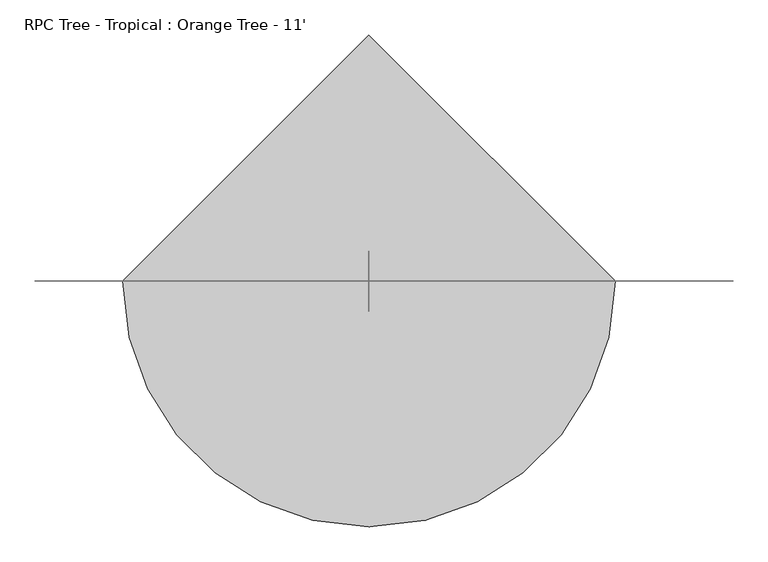
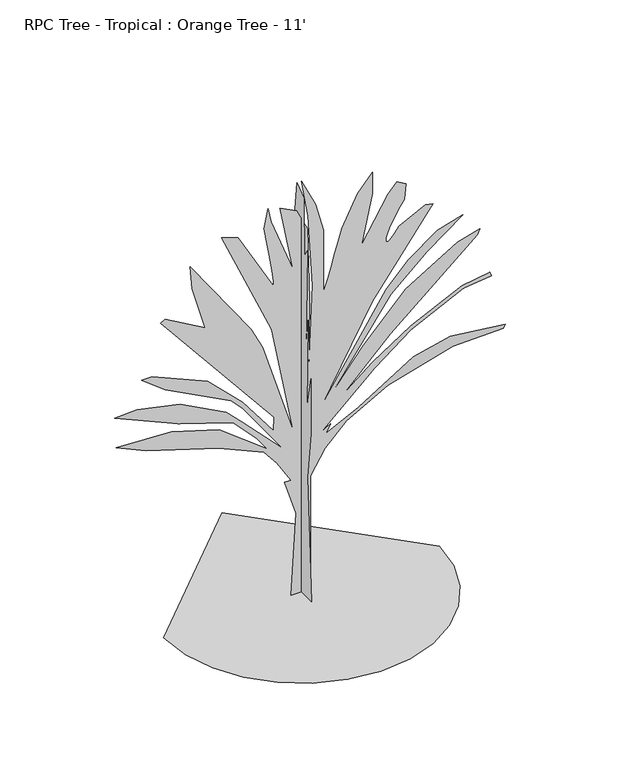
"""IFC4 building model written with IfcOpenShell, lengths in millimetres: geographic element geometry, RPC Tree - Tropical : Orange Tree - 11'."""

from ifc_helpers import new_model, si_unit, origin, place, context, project, spatial, triangles, source, transform, mapped, element, save


def rpc_tree_tropical_orange_tree_11_f00c8d58(model_context):
    return source(origin(), model_context, "Body", "Tessellation", [
        triangles([(-79.3298689, -0.0067032, 0.0519959), (-40.5441867, -0.0067424, 659.3564106), (-131.0442632, -0.0067594, 943.7836716), (-79.3298689, -0.0067591, 939.4744143), (-187.0676514, -0.0067697, 1116.1649374), (-290.4966398, -0.0067774, 1245.4498512), (-639.5662668, -0.0067864, 1396.2829411), (-1199.8044542, -0.0067969, 1572.9734642), (-1432.5167759, -0.0068033, 1680.710202), (-1001.5657551, -0.006802, 1659.1619534), (-635.2570822, -0.0067954, 1547.1160309), (-264.6392246, -0.0067784, 1262.6867352), (-346.5206729, -0.0067853, 1379.043877), (-527.5203807, -0.0067966, 1568.6620995), (-949.8508884, -0.0068049, 1706.56749), (-1445.4466553, -0.006818, 1926.3523304), (-1268.7561321, -0.0068185, 1934.9728798), (-936.9232618, -0.0068141, 1861.7099098), (-583.5422882, -0.0068028, 1672.0916874), (-462.87578, -0.0067956, 1551.4252155), (-143.9727528, -0.0067761, 1223.9016026), (-449.9481534, -0.0068018, 1654.8527687), (-544.7572283, -0.0068077, 1753.973172), (-1053.280549, -0.0068236, 2021.1613689), (-1234.2803295, -0.0068321, 2163.3739094), (-1152.3988449, -0.0068321, 2163.3739094), (-725.7569361, -0.0068208, 1973.7578671), (-454.2573744, -0.0068051, 1710.87682), (-217.2336153, -0.0067861, 1391.9737564), (-212.9248485, -0.0067928, 1504.0196789), (-1087.7564243, -0.0068568, 2577.0796165), (-1053.280549, -0.006858, 2598.6364403), (-742.9959274, -0.0068473, 2417.6280121), (-846.4234079, -0.0068686, 2775.3247833), (-859.3532146, -0.0068794, 2956.3329208), (-389.6149175, -0.0068393, 2284.0318062), (-299.1150636, -0.0068285, 2103.0428535), (-62.092172, -0.0067825, 1331.6405205), (-230.1634038, -0.006836, 2228.0228703), (-618.0202709, -0.0068886, 3111.4647308), (-488.7332133, -0.0068858, 3064.0740189), (-221.54498, -0.0068573, 2585.6979858), (-214.7340586, -0.0068571, 2583.6132294), (-215.6130929, -0.006859, 2614.3043793), (-222.9011473, -0.0068624, 2672.3336861), (-235.3151061, -0.0068672, 2752.1988693), (-251.5719081, -0.0068729, 2848.4845619), (-270.3927252, -0.0068793, 2955.6881927), (-290.4966398, -0.006886, 3068.3725937), (-256.020819, -0.006895, 3219.2055382), (-234.4726067, -0.0068884, 3107.166156), (-66.4013793, -0.0068616, 2658.965316), (-165.5203111, -0.0068935, 3193.3504303), (-36.2349771, -0.0068896, 3128.7014694), (45.6460329, -0.0068791, 2952.0131264), (62.8839478, -0.0068442, 2365.9175056), (54.2648836, -0.0068057, 1719.4951893), (84.4312926, -0.0068508, 2477.9783981), (49.9554582, -0.0068853, 3055.4556496), (2.5507516, -0.006903, 3352.8017441), (110.2884807, -0.0068896, 3128.7014694), (170.6217257, -0.0068758, 2896.0040451), (170.6217257, -0.0068462, 2400.3912735), (174.7678026, -0.0068464, 2403.5505283), (186.3773047, -0.0068483, 2435.660051), (204.2058313, -0.0068517, 2491.8839447), (227.0104713, -0.0068562, 2567.4081139), (253.5448982, -0.0068616, 2657.3965164), (282.5681266, -0.0068675, 2757.056131), (312.835774, -0.0068737, 2861.5090576), (433.5022459, -0.0068881, 3102.8460709), (549.8594968, -0.0068961, 3236.4425674), (549.8594968, -0.0068858, 3064.0740189), (463.6688639, -0.0068624, 2671.9037704), (670.526005, -0.0068827, 3012.3420021), (739.4776829, -0.0068876, 3094.2277016), (808.4292881, -0.006885, 3051.1355644), (795.5016615, -0.0068778, 2930.477813), (763.4244043, -0.0068747, 2878.0580475), (732.8192957, -0.0068717, 2827.0568001), (705.1522345, -0.0068688, 2778.8280579), (681.8954418, -0.0068662, 2734.7903389), (664.5188862, -0.0068639, 2696.3403603), (654.4926813, -0.006862, 2664.8542007), (653.2870136, -0.0068606, 2641.7285774), (659.117835, -0.0068599, 2629.4133408), (668.7915905, -0.0068598, 2628.1884155), (681.6697289, -0.0068603, 2636.183567), (697.1119549, -0.0068612, 2651.5718719), (714.4756479, -0.0068625, 2672.5054779), (733.1202221, -0.0068639, 2697.1356606), (752.4053095, -0.0068655, 2723.6142769), (959.2623779, -0.0068717, 2827.0352898), (1015.2864292, -0.0068709, 2814.1183456), (549.8594968, -0.0068331, 2180.6107933), (144.7647466, -0.0067895, 1447.9978077), (653.2870136, -0.0068367, 2240.939669), (825.6682795, -0.0068475, 2421.9479519), (1049.7622318, -0.0068573, 2585.6979858), (1248.0010036, -0.0068609, 2646.0483719), (972.1921846, -0.0068485, 2439.1848358), (692.074181, -0.0068336, 2189.2291626), (209.4074033, -0.0067928, 1504.0196789), (480.9078552, -0.0068133, 1848.7822105), (804.1201035, -0.0068339, 2193.5491024), (1204.904579, -0.0068483, 2434.864896), (1381.5950294, -0.0068511, 2482.276973), (1360.0469261, -0.0068488, 2443.504921), (687.7628162, -0.0068146, 1870.3282791), (312.835774, -0.0067923, 1495.4011642), (549.8594968, -0.0068036, 1685.0193867), (847.2165281, -0.0068152, 1878.9488285), (1239.3804543, -0.0068265, 2068.5670509), (1459.1673294, -0.0068285, 2103.0428535), (1467.7856987, -0.0068265, 2068.5670509), (1252.3101883, -0.0068249, 2042.7096176), (847.2165281, -0.0068131, 1844.4730259), (567.0963444, -0.0068005, 1633.3067001), (153.3838062, -0.0067776, 1249.7590359), (226.6451048, -0.0067805, 1297.1647179), (192.169502, -0.0067764, 1228.2107872), (442.1206515, -0.0067838, 1353.1865891), (864.4533394, -0.0067997, 1620.3769661), (1153.1918924, -0.0068036, 1685.0193867), (1575.5246166, -0.0068008, 1637.6158848), (1562.5947372, -0.006799, 1607.4492668), (1170.4287764, -0.0067985, 1598.8287174), (670.526005, -0.0067897, 1452.3069923), (347.3115767, -0.0067792, 1275.6164692), (183.5504242, -0.0067694, 1111.8535727), (71.503012, -0.0067584, 926.5446802), (71.503012, -0.0067032, 0.0), (0.038997, 45.6840756, 0.0439303), (0.0389875, -132.7584845, 0.0439196), (0.038997, -82.5717768, 987.0562483), (0.0389875, -127.1825258, 1371.8246956), (0.0389875, -127.1823078, 1817.9322041), (0.038997, -76.995373, 1550.266856), (0.038997, -88.1477446, 2275.1984791), (0.038997, -60.2661842, 2013.1038666), (0.038997, -82.5717768, 2838.4046539), (0.038997, -43.537209, 2771.4776344), (0.038997, -37.9610255, 3239.9028214), (0.0390062, 56.8370831, 3306.8083305), (0.0390062, 112.6004126, 2855.1257263), (0.0390062, 129.3293879, 2208.2713142), (0.0390062, 90.2950426, 1650.6424152), (0.038997, 45.6840756, 948.0219303), (-1065.3657125, 0.0, 0.0487087), (-1037.1999899, -244.1119165, 0.0486943), (-956.9863541, -468.28755, 0.048681), (-831.1488316, -666.1093414, 0.0486691), (-666.1093414, -831.1488316, 0.0486593), (-468.28755, -956.9863541, 0.0486517), (-244.1119165, -1037.1999899, 0.048647), (3.74e-05, -1065.3657125, 0.0486453), (244.1119165, -1037.1999899, 0.048647), (468.28755, -956.9863541, 0.0486517), (666.1093414, -831.1488316, 0.0486593), (831.1488316, -666.1093414, 0.0486691), (956.9863541, -468.28755, 0.048681), (1037.1999899, -244.1119165, 0.0486943), (1065.3657125, 9.31e-05, 0.0487087), (-0.0001494, 1065.3657125, 0.0487723)], [[59, 60, 61], [99, 100, 101], [8, 9, 10], [49, 50, 51], [98, 99, 101], [15, 16, 17], [15, 17, 18], [119, 120, 121], [34, 35, 36], [33, 34, 36], [98, 101, 102], [97, 98, 102], [24, 25, 26], [24, 26, 27], [23, 24, 27], [23, 27, 28], [22, 23, 28], [22, 28, 29], [21, 22, 29], [7, 8, 10], [7, 10, 11], [71, 72, 73], [106, 107, 108], [106, 108, 109], [105, 106, 109], [104, 105, 109], [104, 109, 110], [103, 104, 110], [39, 40, 41], [39, 41, 42], [52, 53, 54], [52, 54, 55], [52, 55, 56], [59, 61, 62], [58, 59, 62], [58, 62, 63], [57, 58, 63], [7, 11, 12], [6, 7, 12], [15, 18, 19], [14, 15, 19], [14, 19, 20], [13, 14, 20], [13, 20, 21], [12, 13, 21], [93, 94, 95], [92, 93, 95], [91, 92, 95], [90, 91, 95], [89, 90, 95], [88, 89, 95], [87, 88, 95], [2, 3, 4], [96, 97, 102], [96, 102, 103], [124, 125, 126], [124, 126, 127], [39, 42, 43], [49, 51, 52], [48, 49, 52], [47, 48, 52], [46, 47, 52], [45, 46, 52], [44, 45, 52], [86, 87, 95], [114, 115, 116], [113, 114, 116], [30, 31, 32], [30, 32, 33], [30, 33, 36], [30, 36, 37], [30, 37, 38], [29, 30, 38], [21, 29, 38], [131, 132, 1], [131, 1, 2], [131, 2, 4], [5, 6, 12], [5, 12, 21], [123, 124, 127], [123, 127, 128], [122, 123, 128], [122, 128, 129], [121, 122, 129], [121, 129, 130], [113, 116, 117], [112, 113, 117], [111, 112, 117], [111, 117, 118], [110, 111, 118], [110, 118, 119], [103, 110, 119], [96, 103, 119], [71, 73, 74], [70, 71, 74], [69, 70, 74], [68, 69, 74], [44, 52, 56], [43, 44, 56], [39, 43, 56], [39, 56, 57], [38, 39, 57], [75, 76, 77], [75, 77, 78], [74, 75, 78], [74, 78, 79], [74, 79, 80], [74, 80, 81], [74, 81, 82], [74, 82, 83], [74, 83, 84], [74, 84, 85], [67, 68, 74], [119, 121, 130], [130, 131, 4], [130, 4, 5], [130, 5, 21], [119, 130, 21], [119, 21, 38], [96, 119, 38], [96, 38, 57], [95, 96, 57], [95, 57, 63], [95, 63, 64], [86, 95, 64], [86, 64, 65], [86, 65, 66], [86, 66, 67], [86, 67, 74], [86, 74, 85], [138, 139, 140], [136, 137, 138], [140, 141, 142], [143, 144, 145], [142, 143, 145], [142, 145, 146], [140, 142, 146], [140, 146, 147], [138, 140, 147], [138, 147, 148], [136, 138, 148], [135, 136, 148], [134, 135, 148], [134, 148, 133], [163, 164, 149], [162, 163, 149], [162, 149, 150], [161, 162, 150], [161, 150, 151], [161, 151, 152], [160, 161, 152], [159, 160, 152], [159, 152, 153], [159, 153, 154], [159, 154, 155], [159, 155, 156], [159, 156, 157], [159, 157, 158]], closed=False),
    ])


if __name__ == "__main__":
    model = new_model("IFC4")
    model_context = context("Model", 3, world=origin())
    ifc_project = project(units=[si_unit("LENGTHUNIT", "METRE", prefix="MILLI")], contexts=[model_context])
    site = spatial("IfcSite", under=ifc_project)
    building = spatial("IfcBuilding", under=site)
    placement = place(None, origin())
    rpc_tree_tropical_orange_tree_11_shape = rpc_tree_tropical_orange_tree_11_f00c8d58(model_context)
    element("IfcGeographicElement", 1, ObjectType="RPC Tree - Tropical : Orange Tree - 11'", at=placement, inside=building, context=model_context, shape_type="MappedRepresentation", body=[
        mapped(rpc_tree_tropical_orange_tree_11_shape, transform((0.0, 0.0, 0.0), x_axis=(1.0, 0.0, 0.0), y_axis=(0.0, 1.0, 0.0), z_axis=(0.0, 0.0, 1.0))),
    ])
    save(model, "model.ifc")

# Revit data of these elements
# Type "RPC Tree - Tropical : Orange Tree - 11'"
#   built-in parameter 1005195 = "RPC-16-G2M6-EAFX-C5H6-W000-ST1L-LVER-AU"
#   Type Comments = "Orange Tree"
#   Assembly Code = "G2050500"
#   Height = 11' - 0"
#   Plan Symbol = element 455245
#   Default Elevation = 0
